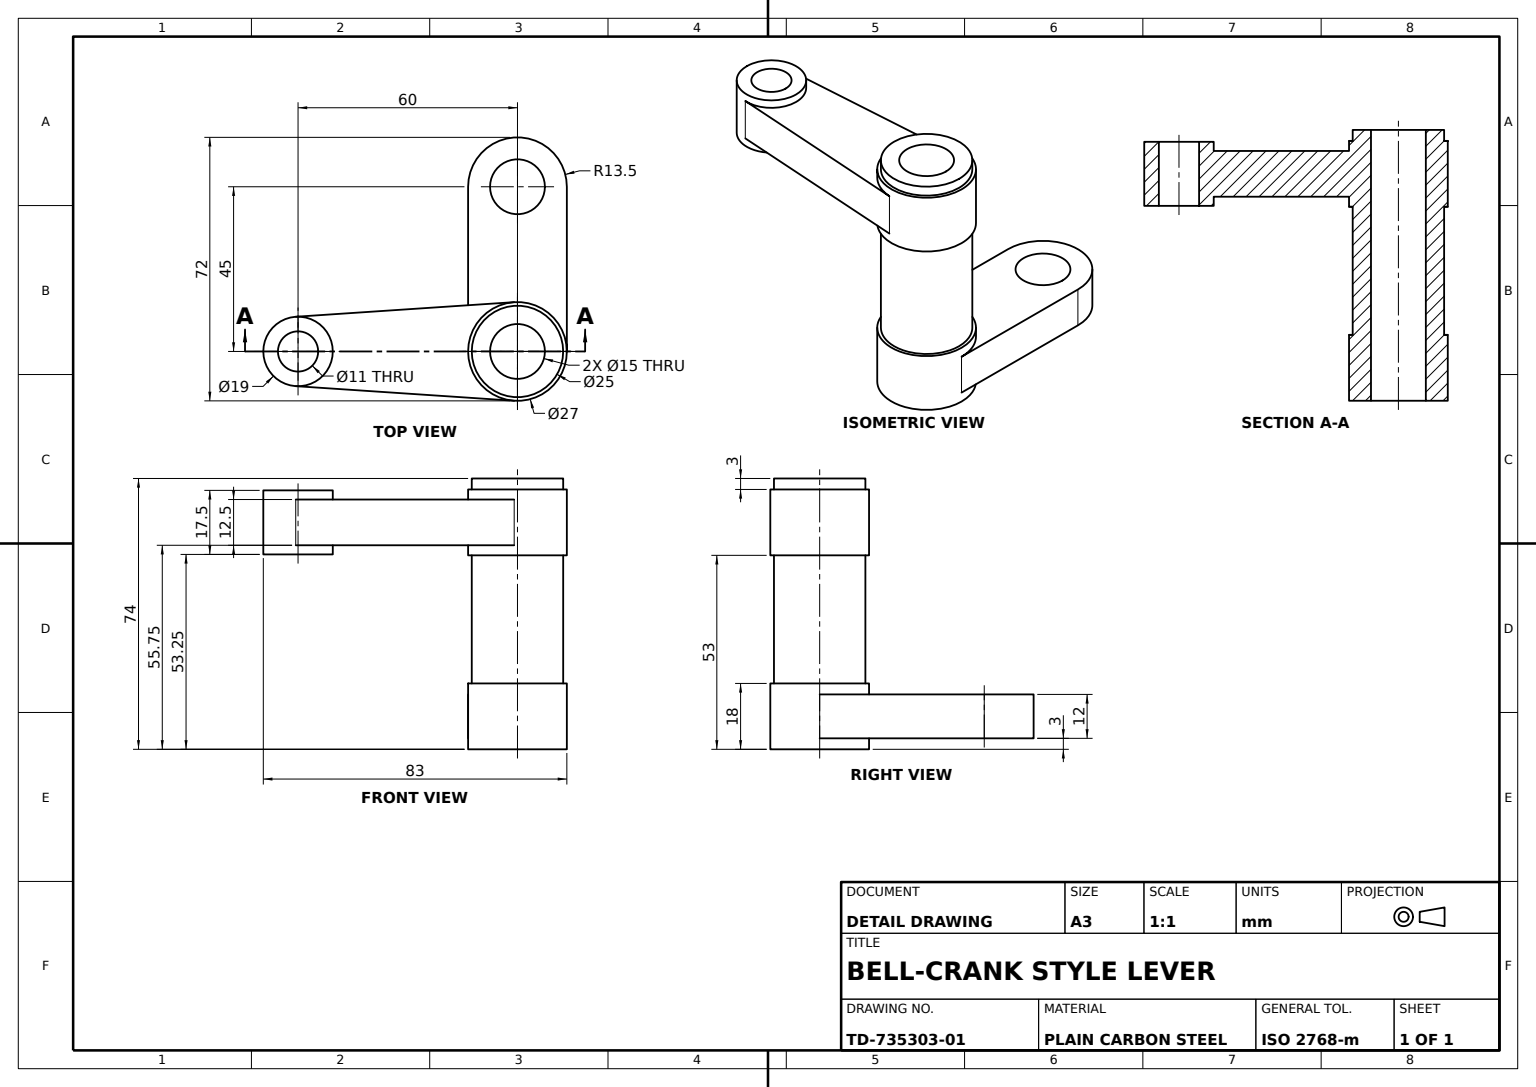
from build123d import *
from build123d.topology import SkipClean

# Parameters (mm, degrees)
LOWER_ARM_SKETCH_R  = 7.5
LOWER_ARM_DEPTH     = 6
HUB_BASE_SKETCH_R   = 13.5
HUB_BASE_BOSS_DEPTH = 9
PIVOT_BORE_SKETCH_R = 7.5
PIVOT_BORE_15_DEPTH = 96.291657557
END_BOSS_SKETCH_R   = 9.5
END_BOSS_SKETCH_R_2 = 5.5
END_BOSS_19_DEPTH   = 8.75
UPPER_ARM_DEPTH     = 6.25


with BuildPart() as part:
    # Lower Arm Sketch → Lower Arm (new, symmetric)
    with BuildSketch(Plane(origin=(0, 0, 0), x_dir=(1, 0, 0), z_dir=(0, 1, 0))):
        with BuildLine():
            Line((-45, 13.5), (0, 13.5))
            ThreePointArc((0, 13.5), (13.5, 0), (0, -13.5))
            Line((0, -13.5), (-45, -13.5))
            ThreePointArc((-45, -13.5), (-58.5, 0), (-45, 13.5))
        make_face()
        with Locations(Location((-45, 0, 0), (0, 0, 270))):
            Circle(LOWER_ARM_SKETCH_R, mode=Mode.SUBTRACT)
    extrude(amount=LOWER_ARM_DEPTH, both=True)

    # Hub Base Sketch → Hub Base Boss (add, symmetric)
    with SkipClean():  # the faces are left unmerged after this step: merging them gives an invalid solid
        with BuildSketch(Plane(origin=(0, 0, 0), x_dir=(1, 0, 0), z_dir=(0, 1, 0))):
            with Locations(Location((0, 0, 0), (0, 0, 270))):
                Circle(HUB_BASE_SKETCH_R)
        extrude(amount=HUB_BASE_BOSS_DEPTH, both=True)

    # Pivot Hub Profile → Pivot Hub (revolve)
    with SkipClean():  # the faces are left unmerged after this step: merging them gives an invalid solid
        with BuildSketch(Plane.XY, mode=Mode.PRIVATE) as pivot_hub_sk:
            Polygon((0, 0), (0, 65), (12.5, 65), (12.5, 62), (13.5, 62), (13.5, 44), (12.5, 44), (12.5, 0), align=None)
        revolve(pivot_hub_sk.sketch.rotate(Axis((0, 0, 0), (0, 1, 0)), 90), axis=Axis((0, 0, 0), (0, 1, 0)))

    # Pivot Bore Sketch → Pivot Bore Ø15 (cut, through all)
    with SkipClean():  # the faces are left unmerged after this step: merging them gives an invalid solid
        with BuildSketch(Plane(origin=(0, 65, 0), x_dir=(1, 0, 0), z_dir=(0, 1, 0))):
            with Locations(Location((0, 0, 0), (0, 0, 270))):
                Circle(PIVOT_BORE_SKETCH_R)
        extrude(amount=-PIVOT_BORE_15_DEPTH, mode=Mode.SUBTRACT)



with BuildPart() as body_2:
    # End Boss Sketch → End Boss Ø19 (new, symmetric)
    with BuildSketch(Plane(origin=(0, 53, 0), x_dir=(1, 0, 0), z_dir=(0, 1, 0))):
        with Locations(Location((0, -60, 0), (0, 0, 270))):
            Circle(END_BOSS_SKETCH_R)
        with Locations(Location((0, -60, 0), (0, 0, 270))):
            Circle(END_BOSS_SKETCH_R_2, mode=Mode.SUBTRACT)
    extrude(amount=END_BOSS_19_DEPTH, both=True)


with BuildPart() as part_1:
    with SkipClean():  # the faces are left unmerged after this step: merging them gives an invalid solid
        add(part.part)

        add(body_2.part)  # Upper Arm merges body 2
        # Upper Arm Sketch → Upper Arm (add, symmetric)
        with BuildSketch(Plane(origin=(0, 53, 0), x_dir=(1, 0, 0), z_dir=(0, 1, 0))):
            with BuildLine():
                Line((13.469966592, -0.9), (9.47886538, -60.633333333))
                ThreePointArc((9.47886538, -60.633333333), (0, -50.5), (-9.47886538, -60.633333333))
                Line((-9.47886538, -60.633333333), (-13.469966592, -0.9))
                ThreePointArc((-13.469966592, -0.9), (0, -13.5), (13.469966592, -0.9))
            make_face()
        extrude(amount=UPPER_ARM_DEPTH, both=True)


solid = part_1.part
